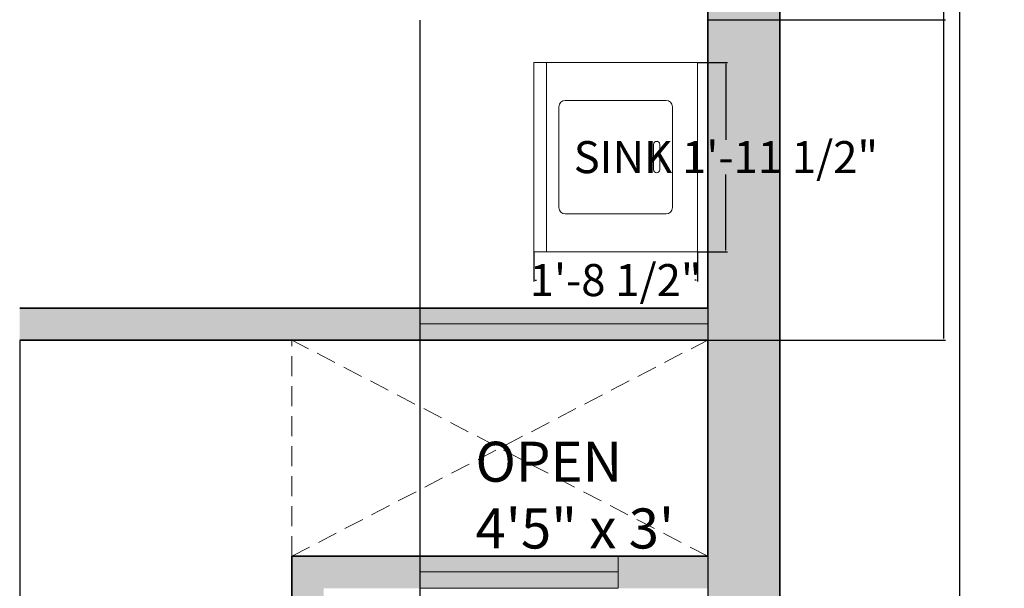
# Model space of a CAD drawing. Units: inches. Extents: x 490 to 851, y 299 to 716.
# Tile 3 of 3: x 728 to 851, y 530 to 601. Entities that reach past the tile are written whole.
import ezdxf

# ---------------------------------------------------------------- set-up
doc = ezdxf.new("R2010")
doc.units = ezdxf.units.IN
doc.header["$MEASUREMENT"] = 0
doc.linetypes.add('DASHED', pattern=[0.75, 0.5, -0.25])
for name, color, linetype, lineweight in [('A-ANNO-DIMS', 2, 'Continuous', 18), ('A-AREA-IDEN', 7, 'Continuous', 25), ('A-EQPM', 8, 'Continuous', 18), ('A-FLOR-OPEN', 7, 'DASHED', 13), ('A-GLAZ', 4, 'Continuous', 18), ('A-GLAZ-PATT', 4, 'Continuous', 13), ('A-WALL', 7, 'Continuous', 35), ('A-WALL-PATT', 1, 'Continuous', 13)]:
    doc.layers.add(name, color=color, linetype=linetype, lineweight=lineweight)
doc.styles.get("Standard").update_dxf_attribs({"font": 'arial.ttf'})
doc.dimstyles.get("Standard").update_dxf_attribs({"dimtxt": 4, "dimasz": 0.18, "dimexe": 0.18, "dimexo": 0.0625, "dimgap": 0.09, "dimtad": 0, "dimtih": 1, "dimtoh": 1, "dimdec": 0, "dimrnd": 6, "dimzin": 0, "dimdsep": 46, "dimlunit": 3, "dimtxsty": 'Standard', "dimcen": 0.09, "dimadec": 0, "dimazin": 0, "dimtfac": 1, "dimtdec": 0, "dimtofl": 0, "dimtmove": 0, "dimatfit": 3, "dimfxl": 1, "dimtolj": 1, "dimtzin": 0, "dimarcsym": 0})

# ---------------------------------------------------------------- blocks, each defined once
blk = doc.blocks.new('LAVAD-01')
for p, q in [((-0.3220654315012172, 0.3584684581579287), (-0.3220654315012172, -0.3915315418420713)), ((0.3279345684987822, 0.3584684581579287), (-0.3220654315012172, 0.3584684581579287)), ((-0.2720654315012174, 0.3584684581579287), (-0.2720654315012174, -0.3915315418420713)), ((0.3279345684987822, -0.3915315418420713), (0.3279345684987822, 0.3584684581579287)), ((0.2029345684987822, 0.2084684581579284), (-0.1970654315012172, 0.2084684581579284)), ((-0.2220654315012176, 0.1834684581579289), (-0.2220654315012176, -0.2165315418420715)), ((0.2279345684987826, -0.2165315418420715), (0.2279345684987826, 0.1834684581579289)), ((0.1654345684987826, 0.0459684581579287), (0.1654345684987826, 0.0459684581579287)), ((0.1529345684987824, 0.0334684581579286), (0.1529345684987824, -0.0665315418420711)), ((0.1779345684987827, -0.0665315418420711), (0.1779345684987827, 0.0334684581579286)), ((0.1654345684987826, -0.0790315418420713), (0.1654345684987826, -0.0790315418420713)), ((-0.1970654315012172, -0.2415315418420709), (0.2029345684987822, -0.2415315418420709)), ((-0.3220654315012172, -0.3915315418420713), (0.3279345684987822, -0.3915315418420713))]:
    blk.add_line(p, q)
for centre, radius, start, end in [((-0.1970654315012172, 0.1834684581579289), 0.025, 90, 180), ((0.2029345684987822, 0.1834684581579289), 0.025, 0, 90), ((0.1654345684987826, 0.0334684581579286), 0.0125, 90, 180), ((0.1654345684987826, 0.0334684581579286), 0.0125, 0, 90), ((0.1654345684987826, -0.0665315418420711), 0.0125, 180, 270), ((0.1654345684987826, -0.0665315418420711), 0.0125, 270, 360), ((-0.1970654315012172, -0.2165315418420715), 0.025, 180, 270), ((0.2029345684987822, -0.2165315418420715), 0.025, 270, 360)]:
    blk.add_arc(centre, radius, start, end)
blk = doc.blocks.new('*D103')
at = {"layer": 'A-ANNO-DIMS', "color": 0, "lineweight": -2, "transparency": 16777216}
for p, q in [((822.7503542437285, 684.9569991519436), (845.3273379142681, 684.9569991519436)), ((845.147337914268, 684.7769991519436), (845.147337914268, 507.0906553593105)), ((845.147337914268, 325.1369991519435), (845.147337914268, 502.8233429445765)), ((822.7503542437283, 324.9569991519435), (845.3273379142681, 324.9569991519435))]:
    blk.add_line(p, q, dxfattribs=at)
at = {"layer": 'A-ANNO-DIMS', "color": 0, "transparency": 16777216}
for points in [[(845.117337914268, 684.7769991519436), (845.1773379142682, 684.7769991519436), (845.147337914268, 684.9569991519436)], [(845.117337914268, 325.1369991519435), (845.1773379142682, 325.1369991519435), (845.147337914268, 324.9569991519435)]]:
    blk.add_solid(points, dxfattribs=at)
at = {"layer": 'Defpoints', "color": 0, "transparency": 16777216}
for p in [(822.6878542437285, 684.9569991519436), (822.6878542437283, 324.9569991519435), (845.147337914268, 324.9569991519435)]:
    blk.add_point(p, dxfattribs=at)
at = {"layer": 'A-ANNO-DIMS', "color": 0, "transparency": 16777216, "insert": (845.147337914268, 504.9569991519431), "char_height": 4, "attachment_point": 5}
blk.add_mtext("\\A1;30'", dxfattribs=at)
blk = doc.blocks.new('*D116')
at = {"layer": 'A-ANNO-DIMS', "color": 0, "lineweight": -2, "transparency": 16777216}
for p, q in [((812.4692901290625, 595.6081943384994), (816.1300972156771, 595.6081943384994)), ((815.9500972156771, 595.4281943384995), (815.9500972156771, 585.9553835404629)), ((815.9500972156771, 572.1661470944048), (815.9500972156771, 581.6389578924412)), ((812.4692901290625, 571.9861470944048), (816.1300972156771, 571.9861470944048))]:
    blk.add_line(p, q, dxfattribs=at)
at = {"layer": 'A-ANNO-DIMS', "color": 0, "transparency": 16777216}
for points in [[(815.9200972156773, 595.4281943384995), (815.9800972156771, 595.4281943384995), (815.9500972156771, 595.6081943384994)], [(815.9200972156773, 572.1661470944048), (815.9800972156771, 572.1661470944048), (815.9500972156771, 571.9861470944048)]]:
    blk.add_solid(points, dxfattribs=at)
at = {"layer": 'Defpoints', "color": 0, "transparency": 16777216}
for p in [(812.4067901290626, 595.6081943384994), (815.9500972156771, 595.6081943384994), (812.4067901290626, 571.9861470944048)]:
    blk.add_point(p, dxfattribs=at)
at = {"layer": 'A-ANNO-DIMS', "color": 0, "transparency": 16777216, "insert": (815.9500972156771, 583.7971707164517), "char_height": 4, "attachment_point": 5}
blk.add_mtext('\\A1;SINK 1\'-11 1/2"', dxfattribs=at)
blk = doc.blocks.new('*D117')
at = {"layer": 'A-ANNO-DIMS', "color": 0, "lineweight": -2, "transparency": 16777216}
for p, q in [((791.9343491841803, 571.9236470944045), (791.9343491841803, 568.2628400077905)), ((812.4067901290622, 571.9236470944045), (812.4067901290622, 568.2628400077905)), ((792.1143491841802, 568.4428400077904), (792.292029411055, 568.4428400077904)), ((812.2267901290624, 568.4428400077904), (812.0491099021872, 568.4428400077904))]:
    blk.add_line(p, q, dxfattribs=at)
at = {"layer": 'A-ANNO-DIMS', "color": 0, "transparency": 16777216}
for points in [[(792.1143491841802, 568.4728400077903), (792.1143491841802, 568.4128400077904), (791.9343491841803, 568.4428400077904)], [(812.2267901290624, 568.4728400077903), (812.2267901290624, 568.4128400077904), (812.4067901290622, 568.4428400077904)]]:
    blk.add_solid(points, dxfattribs=at)
at = {"layer": 'Defpoints', "color": 0, "transparency": 16777216}
for p in [(791.9343491841803, 571.9861470944046), (812.4067901290622, 571.9861470944046), (812.4067901290622, 568.4428400077904)]:
    blk.add_point(p, dxfattribs=at)
at = {"layer": 'A-ANNO-DIMS', "color": 0, "transparency": 16777216, "insert": (802.1705696566211, 568.4428400077904), "char_height": 4, "attachment_point": 5}
blk.add_mtext('\\A1;1\'-8 1/2"', dxfattribs=at)
blk = doc.blocks.new('*D138')
at = {"layer": 'A-ANNO-DIMS', "color": 0, "lineweight": -2, "transparency": 16777216}
for p, q in [((777.687854, 600.8944989999999), (777.687854, 304.927739)), ((813.6878539999999, 600.8944989999999), (813.6878539999999, 304.927739)), ((777.8678539999999, 305.107739), (790.2827107530696, 305.107739)), ((813.507854, 305.107739), (801.0929972469304, 305.107739))]:
    blk.add_line(p, q, dxfattribs=at)
at = {"layer": 'A-ANNO-DIMS', "color": 0, "transparency": 16777216}
for points in [[(777.8678539999999, 305.1377389999999), (777.8678539999999, 305.077739), (777.687854, 305.107739)], [(813.507854, 305.1377389999999), (813.507854, 305.077739), (813.6878539999999, 305.107739)]]:
    blk.add_solid(points, dxfattribs=at)
at = {"layer": 'Defpoints', "color": 0, "transparency": 16777216}
for p in [(777.687854, 600.956999), (813.6878539999999, 600.956999), (813.6878539999999, 305.107739)]:
    blk.add_point(p, dxfattribs=at)
at = {"layer": 'A-ANNO-DIMS', "color": 0, "transparency": 16777216, "insert": (795.6878539999999, 305.107739), "char_height": 4, "attachment_point": 5}
blk.add_mtext('\\A1;3\'-0"', dxfattribs=at)
blk = doc.blocks.new('*D140')
at = {"layer": 'A-ANNO-DIMS', "color": 0, "lineweight": -2, "transparency": 16777216}
for p, q in [((813.7503540000004, 675.9569990000002), (843.3817780000008, 675.9569990000002)), ((843.2017780000009, 675.7769990000002), (843.2017780000009, 640.5906552073671)), ((843.2017780000009, 601.1369990000002), (843.2017780000009, 636.3233427926331)), ((813.7503540000004, 600.9569990000002), (843.3817780000008, 600.9569990000002))]:
    blk.add_line(p, q, dxfattribs=at)
at = {"layer": 'A-ANNO-DIMS', "color": 0, "transparency": 16777216}
for points in [[(843.171778000001, 675.7769990000002), (843.2317780000008, 675.7769990000002), (843.2017780000009, 675.9569990000002)], [(843.171778000001, 601.1369990000002), (843.2317780000008, 601.1369990000002), (843.2017780000009, 600.9569990000002)]]:
    blk.add_solid(points, dxfattribs=at)
at = {"layer": 'Defpoints', "color": 0, "transparency": 16777216}
for p in [(813.6878540000004, 675.9569990000002), (843.2017780000009, 675.9569990000002), (813.6878540000004, 600.9569990000002)]:
    blk.add_point(p, dxfattribs=at)
at = {"layer": 'A-ANNO-DIMS', "color": 0, "transparency": 16777216, "insert": (843.2017780000007, 638.4569989999999), "char_height": 4, "attachment_point": 5}
blk.add_mtext('\\A1;6\'-3"', dxfattribs=at)
blk = doc.blocks.new('*D142')
at = {"layer": 'A-ANNO-DIMS', "color": 0, "lineweight": -2, "transparency": 16777216}
for p, q in [((822.7503540000004, 684.9569990000002), (843.3817780000008, 684.9569990000002)), ((843.2017780000009, 684.7769990000003), (843.2017780000009, 625.089290950887)), ((843.2017780000009, 561.1369990000001), (843.2017780000009, 620.8247070491134)), ((813.7503540000004, 560.9569990000002), (843.3817780000008, 560.9569990000002))]:
    blk.add_line(p, q, dxfattribs=at)
at = {"layer": 'A-ANNO-DIMS', "color": 0, "transparency": 16777216}
for points in [[(843.171778000001, 684.7769990000003), (843.2317780000008, 684.7769990000003), (843.2017780000009, 684.9569990000002)], [(843.171778000001, 561.1369990000001), (843.2317780000008, 561.1369990000001), (843.2017780000009, 560.9569990000002)]]:
    blk.add_solid(points, dxfattribs=at)
at = {"layer": 'Defpoints', "color": 0, "transparency": 16777216}
for p in [(822.6878540000004, 684.9569990000002), (843.2017780000009, 684.9569990000002), (813.6878540000004, 560.9569990000002)]:
    blk.add_point(p, dxfattribs=at)
at = {"layer": 'A-ANNO-DIMS', "color": 0, "transparency": 16777216, "insert": (843.2017780000007, 622.9569989999999), "char_height": 4, "attachment_point": 5}
blk.add_mtext('\\A1;10\'-4"', dxfattribs=at)
blk = doc.blocks.new('*D143')
at = {"layer": 'A-ANNO-DIMS', "color": 0, "lineweight": -2, "transparency": 16777216}
for p, q in [((727.687854, 560.894499), (727.687854, 304.927739)), ((777.687854, 560.894499), (777.687854, 304.927739)), ((727.8678539999999, 305.107739), (747.2008553642565, 305.107739)), ((777.507854, 305.107739), (758.1748526357435, 305.107739))]:
    blk.add_line(p, q, dxfattribs=at)
at = {"layer": 'A-ANNO-DIMS', "color": 0, "transparency": 16777216}
for points in [[(727.8678539999999, 305.1377389999999), (727.8678539999999, 305.077739), (727.687854, 305.107739)], [(777.507854, 305.1377389999999), (777.507854, 305.077739), (777.687854, 305.107739)]]:
    blk.add_solid(points, dxfattribs=at)
at = {"layer": 'Defpoints', "color": 0, "transparency": 16777216}
for p in [(727.687854, 560.9569989999999), (777.687854, 560.9569989999999), (777.687854, 305.107739)]:
    blk.add_point(p, dxfattribs=at)
at = {"layer": 'A-ANNO-DIMS', "color": 0, "transparency": 16777216, "insert": (752.687854, 305.107739), "char_height": 4, "attachment_point": 5}
blk.add_mtext('\\A1;4\'-2"', dxfattribs=at)

msp = doc.modelspace()

# ---------------------------------------------------------------- hatches: boundary and pattern name
at = {"layer": 'A-GLAZ-PATT'}
h = msp.add_hatch(color=256, dxfattribs=at)
h.dxf.hatch_style = 1
h.paths.add_polyline_path([(627.687854243728, 333.9569991519433), (555.7079255371355, 333.9569991519433), (555.7079255371355, 329.1852480156472), (627.687854243728, 329.1852480156472)])
h.paths.add_polyline_path([(627.687854243728, 329.1852480156472), (555.7079255371355, 329.1852480156472), (555.7079255371355, 324.9570274718321), (627.687854243728, 324.9570274718321)])
h.paths.add_polyline_path([(786.3863959033706, 333.8577394632121), (714.3863959033706, 333.8577394632121), (714.3863959033706, 329.0859600070271), (786.3863959033706, 329.0859600070271)])
h.paths.add_polyline_path([(786.3863959033706, 329.0859600070271), (714.3863959033706, 329.0859600070271), (714.3863959033706, 324.9569991519434), (786.3863959033706, 324.9569991519434)])
h.paths.add_polyline_path([(802.5034207310172, 533.9569991519433), (777.7575047331366, 533.9569991519433), (777.7575047331366, 531.99511810472), (802.5034207310172, 531.99511810472)])
h.paths.add_polyline_path([(802.5034207310172, 531.99511810472), (777.7575047331366, 531.99511810472), (777.7575047331366, 529.9710508772687), (802.5034207310172, 529.9710508772687)])
h.paths.add_polyline_path([(813.687854243728, 562.9810663793944), (777.6878542437279, 562.9810663793944), (777.6878542437279, 560.9569991519431), (813.6878542437278, 560.9569991519431)])
h.paths.add_polyline_path([(813.6878542437278, 564.9569991519431), (777.6878542437279, 564.9569991519431), (777.6878542437279, 562.9810663793944), (813.6878542437278, 562.9810663793944)])
at = {"layer": 'A-WALL-PATT'}
h = msp.add_hatch(color=256, dxfattribs=at)
h.dxf.hatch_style = 1
h.paths.add_polyline_path([(555.6878542437281, 497.9569991519433), (611.6878542437282, 497.9569991519434), (611.6878542437281, 493.9569991519433), (615.6878542437281, 493.9569991519433), (615.6878542437281, 501.9569991519433), (555.6878542437281, 501.9569991519433), (555.6878542437281, 529.9569991519433), (651.6878542437281, 529.9569991519433), (651.6878542437281, 533.9569991519433), (555.6878542437281, 533.9569991519433), (555.6878542437281, 675.9569991519433), (813.687854243728, 675.9569991519433), (813.6878542437278, 564.9569991519431), (813.6878542437278, 560.9569991519431), (813.6878542437278, 533.9569991519433), (802.5034207310172, 533.9569991519433), (802.5034207310172, 529.9569991519433), (813.687854243728, 529.9569991519433), (813.687854243728, 465.9569991519433), (727.6878542437282, 465.9569991519433), (727.6878542437282, 461.9569991519433), (813.687854243728, 461.9569991519433), (813.687854243728, 333.9569991519434), (786.3863959033706, 333.9569991519434), (786.3863959033706, 324.9569991519434), (822.687854243728, 324.9569991519434), (822.687854243728, 684.9569991519433), (546.6878542437281, 684.9569991519433), (546.6878542437281, 324.9569991519434), (555.7079255371355, 324.9569991519434), (555.7079255371355, 333.9569991519433), (555.6878542437281, 333.9569991519433), (555.6878542437281, 461.9569991519433), (651.6878542437282, 461.9569991519433), (651.6878542437282, 465.9569991519433), (555.6878542437281, 465.9569991519433)])
h.paths.add_polyline_path([(714.3863959033706, 333.9569991519433), (691.6878542437281, 333.9569991519433), (691.6878542437282, 429.9205150877742), (691.6792956389427, 429.9205150877742), (691.6792956389427, 465.9569991519433), (687.6878542437282, 465.9569991519433), (687.6878542437282, 429.9569991519434), (687.6878542437281, 361.0075905803756), (687.6936932778153, 361.0075905803756), (687.6936932778153, 324.9569991519434), (714.3863959033706, 324.9569991519434)], flags=17)
h.paths.add_polyline_path([(691.6878542437281, 675.9569991519433), (687.6878542437281, 675.9569991519433), (687.6878542437282, 529.9569991519433), (691.6878542437282, 529.9569991519433)], flags=17)
h.paths.add_polyline_path([(777.7575047331366, 533.9569991519433), (761.6878542437282, 533.9569991519433), (761.6878542437282, 497.9569991519433, -0.0312398925164955), (765.6878542437281, 498.2098446269331), (765.6878542437281, 529.9569991519433), (777.7575047331366, 529.9569991519433)], flags=17)
h.paths.add_polyline_path([(777.6878542437279, 564.9569991519434), (727.687854243728, 564.9569991519433), (727.687854243728, 560.9569991519434), (777.6878542437279, 560.9569991519434)], flags=17)

# ---------------------------------------------------------------- linework, layer by layer
at = {"layer": 'A-FLOR-OPEN', "ltscale": 5}
for p, q in [((813.6878542437278, 533.9569991519433), (761.6878542437281, 560.9569991519434)), ((761.6878542437281, 533.9569991519433), (813.687854243728, 560.9569991519434)), ((761.6878542437283, 533.9569991519434), (761.6878542437281, 560.9569991519434))]:
    msp.add_line(p, q, dxfattribs=at)
at = {"layer": 'A-GLAZ'}
for p, q in [((813.6878542437278, 562.9810663793944), (777.6878542437279, 562.9810663793944)), ((802.5034207310172, 529.9710508772687), (802.5034207310172, 533.9710508772687)), ((802.5034207310172, 531.99511810472), (777.7575047331366, 531.99511810472))]:
    msp.add_line(p, q, dxfattribs=at)
msp.add_lwpolyline([(777.6878542437279, 560.9569991519431), (777.6878542437279, 564.9569991519431), (813.6878542437278, 564.9569991519431), (813.6878542437278, 560.9569991519431)], close=True, dxfattribs=at)
msp.add_lwpolyline([(802.5034207310172, 529.9710508772687), (777.7575047331366, 529.9710508772687), (777.7575047331366, 533.9710508772687), (802.5034207310172, 533.9710508772687)], dxfattribs=at)
at = {"layer": 'A-WALL'}
for p, q in [((822.687854243728, 324.9569991519434), (822.687854243728, 684.9569991519433)), ((813.6878542437278, 564.9569991519431), (813.687854243728, 675.9569991519433)), ((813.687854243728, 564.9569991519434), (727.6878542437282, 564.9569991519433)), ((813.687854243728, 560.9569991519434), (727.6878542437282, 560.9569991519434)), ((813.6878542437278, 533.9569991519433), (813.6878542437278, 560.9569991519434)), ((813.687854243728, 533.9569991519433), (761.6878542437282, 533.9569991519433)), ((761.6878542437282, 497.9569991519433), (761.6878542437283, 533.9569991519433))]:
    msp.add_line(p, q, dxfattribs=at)

# ---------------------------------------------------------------- block references
at = {"layer": 'A-EQPM', "xscale": 31.49606299212599, "yscale": 31.49606299212599, "zscale": 31.49606299212599}
msp.add_blockref('LAVAD-01', (802.0781423023288, 584.3178491996667), dxfattribs=at)

# ---------------------------------------------------------------- texts
at = {"layer": 'A-AREA-IDEN', "insert": (784.6468670945559, 548.2613779653489), "char_height": 5, "attachment_point": 1}
msp.add_mtext_dynamic_manual_height_columns('OPEN\\P4\'5" x 3\'', width=54.99209744262703, gutter_width=1, heights=[0], dxfattribs=at)

# ---------------------------------------------------------------- dimensions: what is measured, and where the dimension line sits
at = {"layer": 'A-ANNO-DIMS'}
for base, p1, p2, override, picture, middle in [((843.2017780000009, 684.9569990000002), (813.6878539999999, 560.9569989999999), (822.6878539999999, 684.9569989999999), {"dimdec": 1, "dimlfac": 1, "dimrnd": 0, "dimzin": 1, "dimdsep": 46, "dimlunit": 4, "dimfrac": 2}, '*D142', (843.2017780000007, 622.9569989999999)), ((845.147337914268, 324.9569991519435), (822.687854243728, 684.9569991519433), (822.6878542437278, 324.9569991519434), {"dimclrd": 0, "dimclre": 0, "dimclrt": 0}, '*D103', (845.147337914268, 504.9569991519431)), ((843.2017780000009, 675.9569990000002), (813.6878539999999, 600.956999), (813.6878539999999, 675.956999), {"dimdec": 1, "dimlfac": 1, "dimrnd": 0, "dimzin": 1, "dimdsep": 46, "dimlunit": 4, "dimfrac": 2}, '*D140', (843.2017780000007, 638.4569989999999))]:
    dim = msp.add_linear_dim(base=base, p1=p1, p2=p2, angle=90, dimstyle='Standard', override=override, dxfattribs=at)
    dim.commit()
    dim.dimension.update_dxf_attribs({"geometry": picture, "text_midpoint": middle})
for base, p1, p2, picture, middle in [((813.6878539999999, 305.107739), (777.687854, 600.956999), (813.6878539999999, 600.956999), '*D138', (795.6878539999999, 305.107739)), ((812.4067901290622, 568.4428400077904), (791.9343491841803, 571.9861470944046), (812.4067901290622, 571.9861470944046), '*D117', (802.1705696566211, 568.4428400077904)), ((777.687854, 305.107739), (727.687854, 560.9569989999999), (777.687854, 560.9569989999999), '*D143', (752.687854, 305.107739))]:
    dim = msp.add_linear_dim(base=base, p1=p1, p2=p2, dimstyle='Standard', override={"dimdec": 1, "dimlfac": 1, "dimrnd": 0, "dimzin": 1, "dimdsep": 46, "dimlunit": 4, "dimfrac": 2}, dxfattribs=at)
    dim.commit()
    dim.dimension.update_dxf_attribs({"geometry": picture, "text_midpoint": middle})
dim = msp.add_linear_dim(base=(815.9500972156771, 595.6081943384994), p1=(812.4067901290622, 571.9861470944046), p2=(812.4067901290622, 595.6081943384991), angle=90, text='SINK <>', dimstyle='Standard', override={"dimdec": 1, "dimlfac": 1, "dimrnd": 0, "dimzin": 1, "dimdsep": 46, "dimlunit": 4, "dimfrac": 2}, dxfattribs=at)
dim.commit()
dim.dimension.update_dxf_attribs({"geometry": '*D116', "text_midpoint": (815.9500972156771, 583.7971707164517)})

doc.saveas('drawing.dxf')
